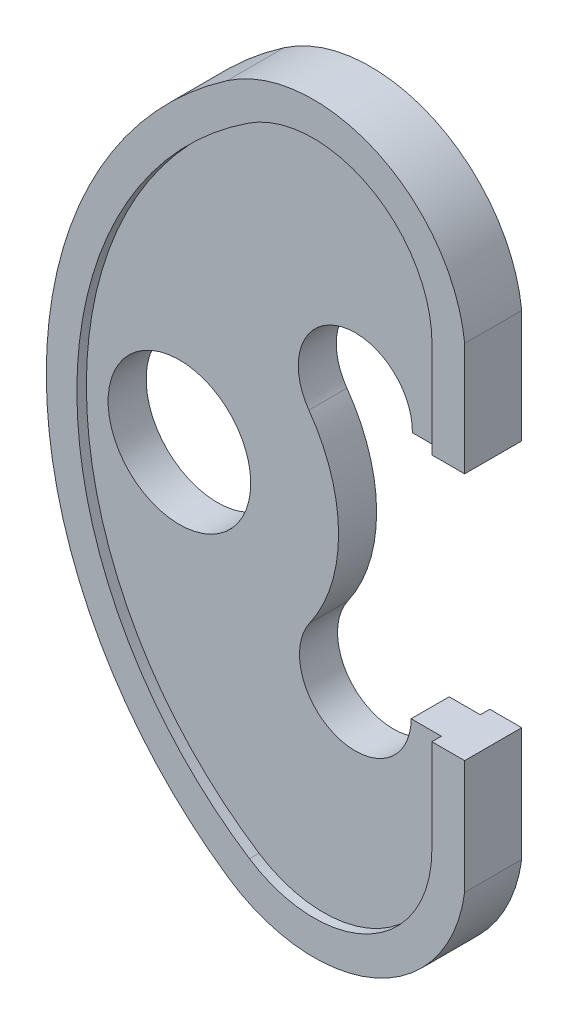
ISO-10303-21;
HEADER;
FILE_DESCRIPTION(('STEP AP214'),'2;1');
FILE_NAME('part.step','',(''),(''),'','','');
FILE_SCHEMA(('AUTOMOTIVE_DESIGN { 1 0 10303 214 1 1 1 1 }'));
ENDSEC;
DATA;
#1=APPLICATION_CONTEXT('core data for automotive mechanical design processes');
#2=APPLICATION_PROTOCOL_DEFINITION('international standard','automotive_design',2000,#1);
#3=PRODUCT_CONTEXT('',#1,'mechanical');
#4=PRODUCT('Part','Part','',(#3));
#5=PRODUCT_RELATED_PRODUCT_CATEGORY('part','',(#4));
#6=PRODUCT_DEFINITION_FORMATION('','',#4);
#7=PRODUCT_DEFINITION_CONTEXT('part definition',#1,'design');
#8=PRODUCT_DEFINITION('design','',#6,#7);
#9=PRODUCT_DEFINITION_SHAPE('','',#8);
#10=(LENGTH_UNIT() NAMED_UNIT(*) SI_UNIT(.MILLI.,.METRE.));
#11=(NAMED_UNIT(*) PLANE_ANGLE_UNIT() SI_UNIT($,.RADIAN.));
#12=(NAMED_UNIT(*) SI_UNIT($,.STERADIAN.) SOLID_ANGLE_UNIT());
#13=UNCERTAINTY_MEASURE_WITH_UNIT(LENGTH_MEASURE(1.E-05),#10,'distance_accuracy_value','');
#14=(GEOMETRIC_REPRESENTATION_CONTEXT(3) GLOBAL_UNCERTAINTY_ASSIGNED_CONTEXT((#13)) GLOBAL_UNIT_ASSIGNED_CONTEXT((#10,
#11,#12)) REPRESENTATION_CONTEXT('',''));
#15=CARTESIAN_POINT('',(0.,0.,0.));
#16=DIRECTION('',(0.,0.,1.));
#17=DIRECTION('',(1.,0.,0.));
#18=AXIS2_PLACEMENT_3D('',#15,#16,#17);
#19=CARTESIAN_POINT('',(-6.87347372301431,8.08028099134121,10.));
#20=DIRECTION('',(0.999999959439754,-0.000284816592779039,0.));
#21=DIRECTION('',(0.000284816592779039,0.999999959439754,0.));
#22=AXIS2_PLACEMENT_3D('',#19,#20,#21);
#23=PLANE('',#22);
#24=DIRECTION('',(0.000284816592779039,0.999999959439753,0.));
#25=VECTOR('',#24,1.);
#26=CARTESIAN_POINT('',(-6.87347372301431,8.08028099134121,10.));
#27=LINE('',#26,#25);
#28=CARTESIAN_POINT('',(-6.8792533227761,-12.2120744187505,10.));
#29=VERTEX_POINT('',#28);
#30=CARTESIAN_POINT('',(-6.87347372301432,8.0802809913412,10.));
#31=VERTEX_POINT('',#30);
#32=EDGE_CURVE('E361',#29,#31,#27,.T.);
#33=ORIENTED_EDGE('',*,*,#32,.F.);
#34=DIRECTION('',(0.,0.,1.));
#35=VECTOR('',#34,1.);
#36=CARTESIAN_POINT('',(-6.8792533227761,-12.2120744187505,9.99999999999997));
#37=LINE('',#36,#35);
#38=CARTESIAN_POINT('',(-6.8792533227761,-12.2120744187505,12.));
#39=VERTEX_POINT('',#38);
#40=EDGE_CURVE('E210',#29,#39,#37,.T.);
#41=ORIENTED_EDGE('',*,*,#40,.T.);
#42=DIRECTION('',(0.000284816592779039,0.999999959439753,0.));
#43=VECTOR('',#42,1.);
#44=CARTESIAN_POINT('',(-6.87347372301431,8.08028099134121,12.));
#45=LINE('',#44,#43);
#46=CARTESIAN_POINT('',(-6.87347372301432,8.0802809913412,12.));
#47=VERTEX_POINT('',#46);
#48=EDGE_CURVE('E224',#39,#47,#45,.T.);
#49=ORIENTED_EDGE('',*,*,#48,.T.);
#50=DIRECTION('',(0.,0.,1.));
#51=VECTOR('',#50,1.);
#52=CARTESIAN_POINT('',(-6.87347372301432,8.0802809913412,10.));
#53=LINE('',#52,#51);
#54=EDGE_CURVE('E234',#31,#47,#53,.T.);
#55=ORIENTED_EDGE('',*,*,#54,.F.);
#56=EDGE_LOOP('',(#33,#41,#49,#55));
#57=FACE_BOUND('',#56,.T.);
#58=ADVANCED_FACE('F50',(#57),#23,.F.);
#59=CARTESIAN_POINT('',(0.,0.,12.));
#60=DIRECTION('',(1.,0.,0.));
#61=DIRECTION('',(0.,1.,0.));
#62=AXIS2_PLACEMENT_3D('',#59,#60,#61);
#63=PLANE('',#62);
#64=DIRECTION('',(0.,-1.,0.));
#65=VECTOR('',#64,1.);
#66=CARTESIAN_POINT('',(0.,0.,12.));
#67=LINE('',#66,#65);
#68=CARTESIAN_POINT('',(0.,11.5582529857865,12.));
#69=VERTEX_POINT('',#68);
#70=CARTESIAN_POINT('',(0.,-12.2120744187505,12.));
#71=VERTEX_POINT('',#70);
#72=EDGE_CURVE('E247',#69,#71,#67,.T.);
#73=ORIENTED_EDGE('',*,*,#72,.T.);
#74=DIRECTION('',(0.,0.,1.));
#75=VECTOR('',#74,1.);
#76=CARTESIAN_POINT('',(0.,-12.2120744187505,0.));
#77=LINE('',#76,#75);
#78=CARTESIAN_POINT('',(0.,-12.2120744187505,0.));
#79=VERTEX_POINT('',#78);
#80=EDGE_CURVE('E313',#79,#71,#77,.T.);
#81=ORIENTED_EDGE('',*,*,#80,.F.);
#82=DIRECTION('',(0.,-1.,0.));
#83=VECTOR('',#82,1.);
#84=CARTESIAN_POINT('',(0.,0.,0.));
#85=LINE('',#84,#83);
#86=CARTESIAN_POINT('',(0.,11.5582529857865,0.));
#87=VERTEX_POINT('',#86);
#88=EDGE_CURVE('E262',#87,#79,#85,.T.);
#89=ORIENTED_EDGE('',*,*,#88,.F.);
#90=DIRECTION('',(0.,0.,-1.));
#91=VECTOR('',#90,1.);
#92=CARTESIAN_POINT('',(0.,11.5582529857865,12.));
#93=LINE('',#92,#91);
#94=EDGE_CURVE('E269',#69,#87,#93,.T.);
#95=ORIENTED_EDGE('',*,*,#94,.F.);
#96=EDGE_LOOP('',(#73,#81,#89,#95));
#97=FACE_BOUND('',#96,.T.);
#98=ADVANCED_FACE('F438',(#97),#63,.T.);
#99=CARTESIAN_POINT('',(-6.71169551772124,8.08738367263815,2.));
#100=DIRECTION('',(1.,0.,0.));
#101=DIRECTION('',(0.,1.,0.));
#102=AXIS2_PLACEMENT_3D('',#99,#100,#101);
#103=PLANE('',#102);
#104=DIRECTION('',(0.,-1.,0.));
#105=VECTOR('',#104,1.);
#106=CARTESIAN_POINT('',(-6.71169551772124,8.08738367263815,0.));
#107=LINE('',#106,#105);
#108=CARTESIAN_POINT('',(-6.71169551772124,8.08738367263815,0.));
#109=VERTEX_POINT('',#108);
#110=CARTESIAN_POINT('',(-6.71169551772125,-12.2120744187505,0.));
#111=VERTEX_POINT('',#110);
#112=EDGE_CURVE('E347',#109,#111,#107,.T.);
#113=ORIENTED_EDGE('',*,*,#112,.T.);
#114=DIRECTION('',(0.,0.,1.));
#115=VECTOR('',#114,1.);
#116=CARTESIAN_POINT('',(-6.71169551772125,-12.2120744187505,2.));
#117=LINE('',#116,#115);
#118=CARTESIAN_POINT('',(-6.71169551772125,-12.2120744187505,2.));
#119=VERTEX_POINT('',#118);
#120=EDGE_CURVE('E281',#111,#119,#117,.T.);
#121=ORIENTED_EDGE('',*,*,#120,.T.);
#122=DIRECTION('',(0.,-1.,0.));
#123=VECTOR('',#122,1.);
#124=CARTESIAN_POINT('',(-6.71169551772124,8.08738367263815,2.));
#125=LINE('',#124,#123);
#126=CARTESIAN_POINT('',(-6.71169551772124,8.08738367263815,2.));
#127=VERTEX_POINT('',#126);
#128=EDGE_CURVE('E333',#127,#119,#125,.T.);
#129=ORIENTED_EDGE('',*,*,#128,.F.);
#130=DIRECTION('',(0.,0.,-1.));
#131=VECTOR('',#130,1.);
#132=CARTESIAN_POINT('',(-6.71169551772124,8.08738367263815,2.));
#133=LINE('',#132,#131);
#134=EDGE_CURVE('E353',#127,#109,#133,.T.);
#135=ORIENTED_EDGE('',*,*,#134,.T.);
#136=EDGE_LOOP('',(#113,#121,#129,#135));
#137=FACE_BOUND('',#136,.T.);
#138=ADVANCED_FACE('F421',(#137),#103,.F.);
#139=CARTESIAN_POINT('',(-62.,-38.4417470142135,0.));
#140=DIRECTION('',(0.,0.,1.));
#141=DIRECTION('',(1.,0.,0.));
#142=AXIS2_PLACEMENT_3D('',#139,#140,#141);
#143=CYLINDRICAL_SURFACE('',#142,15.);
#144=CARTESIAN_POINT('',(-62.,-38.4417470142135,2.));
#145=DIRECTION('',(0.,0.,1.));
#146=DIRECTION('',(1.,0.,0.));
#147=AXIS2_PLACEMENT_3D('',#144,#145,#146);
#148=CIRCLE('',#147,15.);
#149=CARTESIAN_POINT('',(-47.,-38.4417470142135,2.));
#150=VERTEX_POINT('',#149);
#151=EDGE_CURVE('E279',#150,#150,#148,.F.);
#152=ORIENTED_EDGE('',*,*,#151,.T.);
#153=EDGE_LOOP('',(#152));
#154=FACE_BOUND('',#153,.T.);
#155=CARTESIAN_POINT('',(-62.,-38.4417470142135,10.));
#156=DIRECTION('',(0.,0.,1.));
#157=DIRECTION('',(1.,0.,0.));
#158=AXIS2_PLACEMENT_3D('',#155,#156,#157);
#159=CIRCLE('',#158,15.);
#160=CARTESIAN_POINT('',(-47.,-38.4417470142135,10.));
#161=VERTEX_POINT('',#160);
#162=EDGE_CURVE('E231',#161,#161,#159,.F.);
#163=ORIENTED_EDGE('',*,*,#162,.F.);
#164=EDGE_LOOP('',(#163));
#165=FACE_BOUND('',#164,.T.);
#166=ADVANCED_FACE('F594',(#154,#165),#143,.F.);
#167=CARTESIAN_POINT('',(0.,-38.,12.));
#168=DIRECTION('',(0.,0.,-1.));
#169=DIRECTION('',(-1.,0.,0.));
#170=AXIS2_PLACEMENT_3D('',#167,#168,#169);
#171=CYLINDRICAL_SURFACE('',#170,88.);
#172=CARTESIAN_POINT('',(0.,-38.,0.));
#173=DIRECTION('',(0.,0.,1.));
#174=DIRECTION('',(1.,0.,0.));
#175=AXIS2_PLACEMENT_3D('',#172,#173,#174);
#176=CIRCLE('',#175,88.);
#177=CARTESIAN_POINT('',(-49.9890439040348,34.4230314855742,0.));
#178=VERTEX_POINT('',#177);
#179=CARTESIAN_POINT('',(-49.8326643849906,-110.530721492985,0.));
#180=VERTEX_POINT('',#179);
#181=EDGE_CURVE('E251',#178,#180,#176,.T.);
#182=ORIENTED_EDGE('',*,*,#181,.T.);
#183=DIRECTION('',(0.,0.,-1.));
#184=VECTOR('',#183,1.);
#185=CARTESIAN_POINT('',(-49.8326643849906,-110.530721492985,12.));
#186=LINE('',#185,#184);
#187=CARTESIAN_POINT('',(-49.8326643849906,-110.530721492985,12.));
#188=VERTEX_POINT('',#187);
#189=EDGE_CURVE('E275',#188,#180,#186,.T.);
#190=ORIENTED_EDGE('',*,*,#189,.F.);
#191=CARTESIAN_POINT('',(0.,-38.,12.));
#192=DIRECTION('',(0.,0.,1.));
#193=DIRECTION('',(1.,0.,0.));
#194=AXIS2_PLACEMENT_3D('',#191,#192,#193);
#195=CIRCLE('',#194,88.);
#196=CARTESIAN_POINT('',(-49.9890439040348,34.4230314855742,12.));
#197=VERTEX_POINT('',#196);
#198=EDGE_CURVE('E245',#197,#188,#195,.T.);
#199=ORIENTED_EDGE('',*,*,#198,.F.);
#200=DIRECTION('',(0.,0.,-1.));
#201=VECTOR('',#200,1.);
#202=CARTESIAN_POINT('',(-49.9890439040348,34.4230314855742,12.));
#203=LINE('',#202,#201);
#204=EDGE_CURVE('E254',#197,#178,#203,.T.);
#205=ORIENTED_EDGE('',*,*,#204,.T.);
#206=EDGE_LOOP('',(#182,#190,#199,#205));
#207=FACE_BOUND('',#206,.T.);
#208=ADVANCED_FACE('F47',(#207),#171,.T.);
#209=CARTESIAN_POINT('',(-31.7116955177213,-84.1559136773538,12.));
#210=DIRECTION('',(0.,0.,-1.));
#211=DIRECTION('',(-1.,0.,0.));
#212=AXIS2_PLACEMENT_3D('',#209,#210,#211);
#213=CYLINDRICAL_SURFACE('',#212,32.);
#214=CARTESIAN_POINT('',(-31.7116955177213,-84.1559136773538,0.));
#215=DIRECTION('',(0.,0.,1.));
#216=DIRECTION('',(1.,0.,0.));
#217=AXIS2_PLACEMENT_3D('',#214,#215,#216);
#218=CIRCLE('',#217,32.);
#219=CARTESIAN_POINT('',(0.,-88.4417470142135,0.));
#220=VERTEX_POINT('',#219);
#221=EDGE_CURVE('E260',#180,#220,#218,.T.);
#222=ORIENTED_EDGE('',*,*,#221,.T.);
#223=DIRECTION('',(0.,0.,-1.));
#224=VECTOR('',#223,1.);
#225=CARTESIAN_POINT('',(0.,-88.4417470142135,12.));
#226=LINE('',#225,#224);
#227=CARTESIAN_POINT('',(0.,-88.4417470142135,12.));
#228=VERTEX_POINT('',#227);
#229=EDGE_CURVE('E266',#228,#220,#226,.T.);
#230=ORIENTED_EDGE('',*,*,#229,.F.);
#231=CARTESIAN_POINT('',(-31.7116955177213,-84.1559136773538,12.));
#232=DIRECTION('',(0.,0.,1.));
#233=DIRECTION('',(1.,0.,0.));
#234=AXIS2_PLACEMENT_3D('',#231,#232,#233);
#235=CIRCLE('',#234,32.);
#236=EDGE_CURVE('E244',#188,#228,#235,.T.);
#237=ORIENTED_EDGE('',*,*,#236,.F.);
#238=ORIENTED_EDGE('',*,*,#189,.T.);
#239=EDGE_LOOP('',(#222,#230,#237,#238));
#240=FACE_BOUND('',#239,.T.);
#241=ADVANCED_FACE('F534',(#240),#213,.T.);
#242=DIRECTION('',(0.,0.,1.));
#243=VECTOR('',#242,1.);
#244=CARTESIAN_POINT('',(0.,-64.4417470142135,0.));
#245=LINE('',#244,#243);
#246=CARTESIAN_POINT('',(0.,-64.4417470142135,0.));
#247=VERTEX_POINT('',#246);
#248=CARTESIAN_POINT('',(0.,-64.4417470142135,12.));
#249=VERTEX_POINT('',#248);
#250=EDGE_CURVE('E316',#247,#249,#245,.T.);
#251=ORIENTED_EDGE('',*,*,#250,.T.);
#252=EDGE_CURVE('E203',#249,#228,#67,.T.);
#253=ORIENTED_EDGE('',*,*,#252,.T.);
#254=ORIENTED_EDGE('',*,*,#229,.T.);
#255=EDGE_CURVE('E258',#247,#220,#85,.T.);
#256=ORIENTED_EDGE('',*,*,#255,.F.);
#257=EDGE_LOOP('',(#251,#253,#254,#256));
#258=FACE_BOUND('',#257,.T.);
#259=ADVANCED_FACE('F447',(#258),#63,.T.);
#260=CARTESIAN_POINT('',(-31.8112097571131,8.08738367263816,12.));
#261=DIRECTION('',(0.,0.,-1.));
#262=DIRECTION('',(-1.,0.,0.));
#263=AXIS2_PLACEMENT_3D('',#260,#261,#262);
#264=CYLINDRICAL_SURFACE('',#263,32.);
#265=CARTESIAN_POINT('',(-31.8112097571131,8.08738367263816,0.));
#266=DIRECTION('',(0.,0.,1.));
#267=DIRECTION('',(1.,0.,0.));
#268=AXIS2_PLACEMENT_3D('',#265,#266,#267);
#269=CIRCLE('',#268,32.);
#270=EDGE_CURVE('E246',#87,#178,#269,.T.);
#271=ORIENTED_EDGE('',*,*,#270,.T.);
#272=ORIENTED_EDGE('',*,*,#204,.F.);
#273=CARTESIAN_POINT('',(-31.8112097571131,8.08738367263816,12.));
#274=DIRECTION('',(0.,0.,1.));
#275=DIRECTION('',(1.,0.,0.));
#276=AXIS2_PLACEMENT_3D('',#273,#274,#275);
#277=CIRCLE('',#276,32.);
#278=EDGE_CURVE('E252',#69,#197,#277,.T.);
#279=ORIENTED_EDGE('',*,*,#278,.F.);
#280=ORIENTED_EDGE('',*,*,#94,.T.);
#281=EDGE_LOOP('',(#271,#272,#279,#280));
#282=FACE_BOUND('',#281,.T.);
#283=ADVANCED_FACE('F519',(#282),#264,.T.);
#284=CARTESIAN_POINT('',(0.,0.,12.));
#285=DIRECTION('',(0.,0.,1.));
#286=DIRECTION('',(1.,0.,0.));
#287=AXIS2_PLACEMENT_3D('',#284,#285,#286);
#288=PLANE('',#287);
#289=ORIENTED_EDGE('',*,*,#48,.F.);
#290=DIRECTION('',(-1.,0.,0.));
#291=VECTOR('',#290,1.);
#292=CARTESIAN_POINT('',(0.,-12.2120744187505,12.));
#293=LINE('',#292,#291);
#294=EDGE_CURVE('E207',#71,#39,#293,.T.);
#295=ORIENTED_EDGE('',*,*,#294,.F.);
#296=ORIENTED_EDGE('',*,*,#72,.F.);
#297=ORIENTED_EDGE('',*,*,#278,.T.);
#298=ORIENTED_EDGE('',*,*,#198,.T.);
#299=ORIENTED_EDGE('',*,*,#236,.T.);
#300=ORIENTED_EDGE('',*,*,#252,.F.);
#301=DIRECTION('',(1.,0.,0.));
#302=VECTOR('',#301,1.);
#303=CARTESIAN_POINT('',(0.,-64.4417470142135,12.));
#304=LINE('',#303,#302);
#305=CARTESIAN_POINT('',(-6.89412920077007,-64.4417470142135,12.));
#306=VERTEX_POINT('',#305);
#307=EDGE_CURVE('E200',#306,#249,#304,.T.);
#308=ORIENTED_EDGE('',*,*,#307,.F.);
#309=CARTESIAN_POINT('',(-6.89974613553398,-84.1629805325237,12.));
#310=VERTEX_POINT('',#309);
#311=EDGE_CURVE('E205',#310,#306,#45,.T.);
#312=ORIENTED_EDGE('',*,*,#311,.F.);
#313=CARTESIAN_POINT('',(-31.7116955177213,-84.1559136773538,12.));
#314=DIRECTION('',(0.,0.,1.));
#315=DIRECTION('',(1.,0.,0.));
#316=AXIS2_PLACEMENT_3D('',#313,#314,#315);
#317=CIRCLE('',#316,24.8119503885661);
#318=CARTESIAN_POINT('',(-45.2633918891372,-104.940148268544,12.));
#319=VERTEX_POINT('',#318);
#320=EDGE_CURVE('E227',#319,#310,#317,.T.);
#321=ORIENTED_EDGE('',*,*,#320,.F.);
#322=CARTESIAN_POINT('',(-1.56929719947238,-37.9265221224338,12.));
#323=DIRECTION('',(0.,0.,1.));
#324=DIRECTION('',(1.,0.,0.));
#325=AXIS2_PLACEMENT_3D('',#322,#323,#324);
#326=CIRCLE('',#325,79.9999999999999);
#327=CARTESIAN_POINT('',(-45.5077929095733,28.9271134909974,12.));
#328=VERTEX_POINT('',#327);
#329=EDGE_CURVE('E282',#328,#319,#326,.T.);
#330=ORIENTED_EDGE('',*,*,#329,.F.);
#331=CARTESIAN_POINT('',(-31.8112097571131,8.08738367263816,12.));
#332=DIRECTION('',(0.,0.,1.));
#333=DIRECTION('',(1.,0.,0.));
#334=AXIS2_PLACEMENT_3D('',#331,#332,#333);
#335=CIRCLE('',#334,24.9377370455795);
#336=EDGE_CURVE('E222',#47,#328,#335,.T.);
#337=ORIENTED_EDGE('',*,*,#336,.F.);
#338=EDGE_LOOP('',(#289,#295,#296,#297,#298,#299,#300,#308,#312,#321,#330,#337));
#339=FACE_BOUND('',#338,.T.);
#340=ADVANCED_FACE('F198',(#339),#288,.T.);
#341=CARTESIAN_POINT('',(0.,0.,0.));
#342=DIRECTION('',(0.,0.,1.));
#343=DIRECTION('',(1.,0.,0.));
#344=AXIS2_PLACEMENT_3D('',#341,#342,#343);
#345=PLANE('',#344);
#346=ORIENTED_EDGE('',*,*,#88,.T.);
#347=DIRECTION('',(-1.,0.,0.));
#348=VECTOR('',#347,1.);
#349=CARTESIAN_POINT('',(0.,-12.2120744187505,0.));
#350=LINE('',#349,#348);
#351=EDGE_CURVE('E324',#79,#111,#350,.T.);
#352=ORIENTED_EDGE('',*,*,#351,.T.);
#353=ORIENTED_EDGE('',*,*,#112,.F.);
#354=CARTESIAN_POINT('',(-31.8112097571131,8.08738367263816,0.));
#355=DIRECTION('',(0.,0.,-1.));
#356=DIRECTION('',(-1.,0.,0.));
#357=AXIS2_PLACEMENT_3D('',#354,#355,#356);
#358=CIRCLE('',#357,25.0995142393918);
#359=CARTESIAN_POINT('',(-45.4907300450156,29.1315358234447,0.));
#360=VERTEX_POINT('',#359);
#361=EDGE_CURVE('E345',#360,#109,#358,.T.);
#362=ORIENTED_EDGE('',*,*,#361,.F.);
#363=CARTESIAN_POINT('',(-1.88982157346105,-37.9427571691402,0.));
#364=DIRECTION('',(0.,0.,-1.));
#365=DIRECTION('',(1.,0.,0.));
#366=AXIS2_PLACEMENT_3D('',#363,#364,#365);
#367=CIRCLE('',#366,80.);
#368=CARTESIAN_POINT('',(-45.2670927651123,-105.16189390836,0.));
#369=VERTEX_POINT('',#368);
#370=EDGE_CURVE('E68',#369,#360,#367,.T.);
#371=ORIENTED_EDGE('',*,*,#370,.F.);
#372=CARTESIAN_POINT('',(-31.7116955177213,-84.1559136773538,0.));
#373=DIRECTION('',(0.,0.,-1.));
#374=DIRECTION('',(-1.,0.,0.));
#375=AXIS2_PLACEMENT_3D('',#372,#373,#374);
#376=CIRCLE('',#375,25.);
#377=CARTESIAN_POINT('',(-6.71169551772124,-84.1559136773538,0.));
#378=VERTEX_POINT('',#377);
#379=EDGE_CURVE('E332',#378,#369,#376,.T.);
#380=ORIENTED_EDGE('',*,*,#379,.F.);
#381=CARTESIAN_POINT('',(-6.71169551772125,-64.4417470142135,0.));
#382=VERTEX_POINT('',#381);
#383=EDGE_CURVE('E343',#382,#378,#107,.T.);
#384=ORIENTED_EDGE('',*,*,#383,.F.);
#385=DIRECTION('',(1.,0.,0.));
#386=VECTOR('',#385,1.);
#387=CARTESIAN_POINT('',(-13.25855129318,-64.4417470142135,0.));
#388=LINE('',#387,#386);
#389=EDGE_CURVE('E65',#382,#247,#388,.T.);
#390=ORIENTED_EDGE('',*,*,#389,.T.);
#391=ORIENTED_EDGE('',*,*,#255,.T.);
#392=ORIENTED_EDGE('',*,*,#221,.F.);
#393=ORIENTED_EDGE('',*,*,#181,.F.);
#394=ORIENTED_EDGE('',*,*,#270,.F.);
#395=EDGE_LOOP('',(#346,#352,#353,#362,#371,#380,#384,#390,#391,#392,#393,#394));
#396=FACE_BOUND('',#395,.T.);
#397=ADVANCED_FACE('F433',(#396),#345,.F.);
#398=CARTESIAN_POINT('',(-1.56929719947238,-37.9265221224338,10.));
#399=DIRECTION('',(0.,0.,1.));
#400=DIRECTION('',(1.,0.,0.));
#401=AXIS2_PLACEMENT_3D('',#398,#399,#400);
#402=PLANE('',#401);
#403=DIRECTION('',(-1.,0.,0.));
#404=VECTOR('',#403,1.);
#405=CARTESIAN_POINT('',(-12.9979710146966,-12.2120744187505,10.));
#406=LINE('',#405,#404);
#407=CARTESIAN_POINT('',(-12.9979710146966,-12.2120744187505,10.));
#408=VERTEX_POINT('',#407);
#409=EDGE_CURVE('E397',#29,#408,#406,.T.);
#410=ORIENTED_EDGE('',*,*,#409,.F.);
#411=ORIENTED_EDGE('',*,*,#32,.T.);
#412=CARTESIAN_POINT('',(-31.8112097571131,8.08738367263816,10.));
#413=DIRECTION('',(0.,0.,1.));
#414=DIRECTION('',(1.,0.,0.));
#415=AXIS2_PLACEMENT_3D('',#412,#413,#414);
#416=CIRCLE('',#415,24.9377370455795);
#417=CARTESIAN_POINT('',(-45.5077929095733,28.9271134909974,10.));
#418=VERTEX_POINT('',#417);
#419=EDGE_CURVE('E241',#31,#418,#416,.T.);
#420=ORIENTED_EDGE('',*,*,#419,.T.);
#421=CARTESIAN_POINT('',(-1.56929719947238,-37.9265221224338,10.));
#422=DIRECTION('',(0.,0.,1.));
#423=DIRECTION('',(1.,0.,0.));
#424=AXIS2_PLACEMENT_3D('',#421,#422,#423);
#425=CIRCLE('',#424,79.9999999999999);
#426=CARTESIAN_POINT('',(-45.2633918891372,-104.940148268544,10.));
#427=VERTEX_POINT('',#426);
#428=EDGE_CURVE('E223',#418,#427,#425,.T.);
#429=ORIENTED_EDGE('',*,*,#428,.T.);
#430=CARTESIAN_POINT('',(-31.7116955177213,-84.1559136773538,10.));
#431=DIRECTION('',(0.,0.,1.));
#432=DIRECTION('',(1.,0.,0.));
#433=AXIS2_PLACEMENT_3D('',#430,#431,#432);
#434=CIRCLE('',#433,24.8119503885661);
#435=CARTESIAN_POINT('',(-6.89974613553398,-84.1629805325237,10.));
#436=VERTEX_POINT('',#435);
#437=EDGE_CURVE('E359',#427,#436,#434,.T.);
#438=ORIENTED_EDGE('',*,*,#437,.T.);
#439=CARTESIAN_POINT('',(-6.89412920077007,-64.4417470142135,10.));
#440=VERTEX_POINT('',#439);
#441=EDGE_CURVE('E364',#436,#440,#27,.T.);
#442=ORIENTED_EDGE('',*,*,#441,.T.);
#443=DIRECTION('',(1.,0.,0.));
#444=VECTOR('',#443,1.);
#445=CARTESIAN_POINT('',(-6.89412920077007,-64.4417470142135,10.));
#446=LINE('',#445,#444);
#447=CARTESIAN_POINT('',(-13.25855129318,-64.4417470142135,10.));
#448=VERTEX_POINT('',#447);
#449=EDGE_CURVE('E214',#448,#440,#446,.T.);
#450=ORIENTED_EDGE('',*,*,#449,.F.);
#451=CARTESIAN_POINT('',(-25.,-64.4417470142135,10.));
#452=DIRECTION('',(0.,0.,1.));
#453=DIRECTION('',(1.,0.,0.));
#454=AXIS2_PLACEMENT_3D('',#451,#452,#453);
#455=CIRCLE('',#454,11.74144870682);
#456=CARTESIAN_POINT('',(-34.6067558410355,-57.6910537205129,10.));
#457=VERTEX_POINT('',#456);
#458=EDGE_CURVE('E389',#457,#448,#455,.T.);
#459=ORIENTED_EDGE('',*,*,#458,.F.);
#460=CARTESIAN_POINT('',(-62.,-38.4417470142135,10.));
#461=DIRECTION('',(0.,0.,-1.));
#462=DIRECTION('',(1.,0.,0.));
#463=AXIS2_PLACEMENT_3D('',#460,#461,#462);
#464=CIRCLE('',#463,33.4802275115601);
#465=CARTESIAN_POINT('',(-34.7596117688961,-18.9767301058068,10.));
#466=VERTEX_POINT('',#465);
#467=EDGE_CURVE('E388',#466,#457,#464,.T.);
#468=ORIENTED_EDGE('',*,*,#467,.F.);
#469=CARTESIAN_POINT('',(-24.9960981051858,-12.0000689460154,10.));
#470=DIRECTION('',(0.,0.,1.));
#471=DIRECTION('',(1.,0.,0.));
#472=AXIS2_PLACEMENT_3D('',#469,#470,#471);
#473=CIRCLE('',#472,12.);
#474=EDGE_CURVE('E308',#408,#466,#473,.T.);
#475=ORIENTED_EDGE('',*,*,#474,.F.);
#476=EDGE_LOOP('',(#410,#411,#420,#429,#438,#442,#450,#459,#468,#475));
#477=FACE_BOUND('',#476,.T.);
#478=ORIENTED_EDGE('',*,*,#162,.T.);
#479=EDGE_LOOP('',(#478));
#480=FACE_BOUND('',#479,.T.);
#481=ADVANCED_FACE('F398',(#477,#480),#402,.T.);
#482=CARTESIAN_POINT('',(-1.56929719947238,-37.9265221224338,10.));
#483=DIRECTION('',(0.,0.,1.));
#484=DIRECTION('',(1.,0.,0.));
#485=AXIS2_PLACEMENT_3D('',#482,#483,#484);
#486=CYLINDRICAL_SURFACE('',#485,79.9999999999999);
#487=ORIENTED_EDGE('',*,*,#329,.T.);
#488=DIRECTION('',(0.,0.,1.));
#489=VECTOR('',#488,1.);
#490=CARTESIAN_POINT('',(-45.2633918891372,-104.940148268544,10.));
#491=LINE('',#490,#489);
#492=EDGE_CURVE('E238',#427,#319,#491,.T.);
#493=ORIENTED_EDGE('',*,*,#492,.F.);
#494=ORIENTED_EDGE('',*,*,#428,.F.);
#495=DIRECTION('',(0.,0.,1.));
#496=VECTOR('',#495,1.);
#497=CARTESIAN_POINT('',(-45.5077929095733,28.9271134909974,10.));
#498=LINE('',#497,#496);
#499=EDGE_CURVE('E233',#418,#328,#498,.T.);
#500=ORIENTED_EDGE('',*,*,#499,.T.);
#501=EDGE_LOOP('',(#487,#493,#494,#500));
#502=FACE_BOUND('',#501,.T.);
#503=ADVANCED_FACE('F424',(#502),#486,.F.);
#504=CARTESIAN_POINT('',(-31.8112097571131,8.08738367263816,10.));
#505=DIRECTION('',(0.,0.,1.));
#506=DIRECTION('',(1.,0.,0.));
#507=AXIS2_PLACEMENT_3D('',#504,#505,#506);
#508=CYLINDRICAL_SURFACE('',#507,24.9377370455795);
#509=ORIENTED_EDGE('',*,*,#336,.T.);
#510=ORIENTED_EDGE('',*,*,#499,.F.);
#511=ORIENTED_EDGE('',*,*,#419,.F.);
#512=ORIENTED_EDGE('',*,*,#54,.T.);
#513=EDGE_LOOP('',(#509,#510,#511,#512));
#514=FACE_BOUND('',#513,.T.);
#515=ADVANCED_FACE('F374',(#514),#508,.F.);
#516=ORIENTED_EDGE('',*,*,#311,.T.);
#517=DIRECTION('',(0.,0.,-1.));
#518=VECTOR('',#517,1.);
#519=CARTESIAN_POINT('',(-6.89412920077007,-64.4417470142135,10.));
#520=LINE('',#519,#518);
#521=EDGE_CURVE('E208',#306,#440,#520,.T.);
#522=ORIENTED_EDGE('',*,*,#521,.T.);
#523=ORIENTED_EDGE('',*,*,#441,.F.);
#524=DIRECTION('',(0.,0.,1.));
#525=VECTOR('',#524,1.);
#526=CARTESIAN_POINT('',(-6.89974613553398,-84.1629805325237,10.));
#527=LINE('',#526,#525);
#528=EDGE_CURVE('E216',#436,#310,#527,.T.);
#529=ORIENTED_EDGE('',*,*,#528,.T.);
#530=EDGE_LOOP('',(#516,#522,#523,#529));
#531=FACE_BOUND('',#530,.T.);
#532=ADVANCED_FACE('F219',(#531),#23,.F.);
#533=CARTESIAN_POINT('',(-31.7116955177213,-84.1559136773538,10.));
#534=DIRECTION('',(0.,0.,1.));
#535=DIRECTION('',(1.,0.,0.));
#536=AXIS2_PLACEMENT_3D('',#533,#534,#535);
#537=CYLINDRICAL_SURFACE('',#536,24.8119503885661);
#538=ORIENTED_EDGE('',*,*,#320,.T.);
#539=ORIENTED_EDGE('',*,*,#528,.F.);
#540=ORIENTED_EDGE('',*,*,#437,.F.);
#541=ORIENTED_EDGE('',*,*,#492,.T.);
#542=EDGE_LOOP('',(#538,#539,#540,#541));
#543=FACE_BOUND('',#542,.T.);
#544=ADVANCED_FACE('F369',(#543),#537,.F.);
#545=CARTESIAN_POINT('',(-1.88982157346105,-37.9427571691402,2.));
#546=DIRECTION('',(0.,0.,1.));
#547=DIRECTION('',(1.,0.,0.));
#548=AXIS2_PLACEMENT_3D('',#545,#546,#547);
#549=PLANE('',#548);
#550=ORIENTED_EDGE('',*,*,#128,.T.);
#551=DIRECTION('',(-1.,0.,0.));
#552=VECTOR('',#551,1.);
#553=CARTESIAN_POINT('',(-1.88982157346103,-12.2120744187505,2.));
#554=LINE('',#553,#552);
#555=CARTESIAN_POINT('',(-12.9979710146966,-12.2120744187505,2.));
#556=VERTEX_POINT('',#555);
#557=EDGE_CURVE('E323',#119,#556,#554,.T.);
#558=ORIENTED_EDGE('',*,*,#557,.T.);
#559=CARTESIAN_POINT('',(-24.9960981051858,-12.0000689460154,2.));
#560=DIRECTION('',(0.,0.,1.));
#561=DIRECTION('',(1.,0.,0.));
#562=AXIS2_PLACEMENT_3D('',#559,#560,#561);
#563=CIRCLE('',#562,12.);
#564=CARTESIAN_POINT('',(-34.7596117688961,-18.9767301058068,2.));
#565=VERTEX_POINT('',#564);
#566=EDGE_CURVE('E11',#556,#565,#563,.T.);
#567=ORIENTED_EDGE('',*,*,#566,.T.);
#568=CARTESIAN_POINT('',(-62.,-38.4417470142135,2.));
#569=DIRECTION('',(0.,0.,1.));
#570=DIRECTION('',(1.,0.,0.));
#571=AXIS2_PLACEMENT_3D('',#568,#569,#570);
#572=CIRCLE('',#571,33.4802275115601);
#573=CARTESIAN_POINT('',(-34.6067558410355,-57.6910537205129,2.));
#574=VERTEX_POINT('',#573);
#575=EDGE_CURVE('E54',#565,#574,#572,.F.);
#576=ORIENTED_EDGE('',*,*,#575,.T.);
#577=CARTESIAN_POINT('',(-25.,-64.4417470142135,2.));
#578=DIRECTION('',(0.,0.,1.));
#579=DIRECTION('',(1.,0.,0.));
#580=AXIS2_PLACEMENT_3D('',#577,#578,#579);
#581=CIRCLE('',#580,11.74144870682);
#582=CARTESIAN_POINT('',(-13.25855129318,-64.4417470142135,2.));
#583=VERTEX_POINT('',#582);
#584=EDGE_CURVE('E289',#574,#583,#581,.T.);
#585=ORIENTED_EDGE('',*,*,#584,.T.);
#586=DIRECTION('',(1.,0.,0.));
#587=VECTOR('',#586,1.);
#588=CARTESIAN_POINT('',(-1.88982157346105,-64.4417470142135,2.));
#589=LINE('',#588,#587);
#590=CARTESIAN_POINT('',(-6.71169551772125,-64.4417470142135,2.));
#591=VERTEX_POINT('',#590);
#592=EDGE_CURVE('E315',#583,#591,#589,.T.);
#593=ORIENTED_EDGE('',*,*,#592,.T.);
#594=CARTESIAN_POINT('',(-6.71169551772124,-84.1559136773538,2.));
#595=VERTEX_POINT('',#594);
#596=EDGE_CURVE('E331',#591,#595,#125,.T.);
#597=ORIENTED_EDGE('',*,*,#596,.T.);
#598=CARTESIAN_POINT('',(-31.7116955177213,-84.1559136773538,2.));
#599=DIRECTION('',(0.,0.,-1.));
#600=DIRECTION('',(-1.,0.,0.));
#601=AXIS2_PLACEMENT_3D('',#598,#599,#600);
#602=CIRCLE('',#601,25.);
#603=CARTESIAN_POINT('',(-45.2670927651123,-105.16189390836,2.));
#604=VERTEX_POINT('',#603);
#605=EDGE_CURVE('E340',#595,#604,#602,.T.);
#606=ORIENTED_EDGE('',*,*,#605,.T.);
#607=CARTESIAN_POINT('',(-1.88982157346105,-37.9427571691402,2.));
#608=DIRECTION('',(0.,0.,-1.));
#609=DIRECTION('',(1.,0.,0.));
#610=AXIS2_PLACEMENT_3D('',#607,#608,#609);
#611=CIRCLE('',#610,80.);
#612=CARTESIAN_POINT('',(-45.4907300450156,29.1315358234447,2.));
#613=VERTEX_POINT('',#612);
#614=EDGE_CURVE('E330',#604,#613,#611,.T.);
#615=ORIENTED_EDGE('',*,*,#614,.T.);
#616=CARTESIAN_POINT('',(-31.8112097571131,8.08738367263816,2.));
#617=DIRECTION('',(0.,0.,-1.));
#618=DIRECTION('',(-1.,0.,0.));
#619=AXIS2_PLACEMENT_3D('',#616,#617,#618);
#620=CIRCLE('',#619,25.0995142393918);
#621=EDGE_CURVE('E328',#613,#127,#620,.T.);
#622=ORIENTED_EDGE('',*,*,#621,.T.);
#623=EDGE_LOOP('',(#550,#558,#567,#576,#585,#593,#597,#606,#615,#622));
#624=FACE_BOUND('',#623,.T.);
#625=ORIENTED_EDGE('',*,*,#151,.F.);
#626=EDGE_LOOP('',(#625));
#627=FACE_BOUND('',#626,.T.);
#628=ADVANCED_FACE('F292',(#624,#627),#549,.F.);
#629=CARTESIAN_POINT('',(-1.88982157346105,-37.9427571691402,2.));
#630=DIRECTION('',(0.,0.,-1.));
#631=DIRECTION('',(-1.,0.,0.));
#632=AXIS2_PLACEMENT_3D('',#629,#630,#631);
#633=CYLINDRICAL_SURFACE('',#632,80.);
#634=ORIENTED_EDGE('',*,*,#370,.T.);
#635=DIRECTION('',(0.,0.,-1.));
#636=VECTOR('',#635,1.);
#637=CARTESIAN_POINT('',(-45.4907300450156,29.1315358234447,2.));
#638=LINE('',#637,#636);
#639=EDGE_CURVE('E338',#613,#360,#638,.T.);
#640=ORIENTED_EDGE('',*,*,#639,.F.);
#641=ORIENTED_EDGE('',*,*,#614,.F.);
#642=DIRECTION('',(0.,0.,-1.));
#643=VECTOR('',#642,1.);
#644=CARTESIAN_POINT('',(-45.2670927651123,-105.16189390836,2.));
#645=LINE('',#644,#643);
#646=EDGE_CURVE('E285',#604,#369,#645,.T.);
#647=ORIENTED_EDGE('',*,*,#646,.T.);
#648=EDGE_LOOP('',(#634,#640,#641,#647));
#649=FACE_BOUND('',#648,.T.);
#650=ADVANCED_FACE('F417',(#649),#633,.F.);
#651=CARTESIAN_POINT('',(-31.7116955177213,-84.1559136773538,2.));
#652=DIRECTION('',(0.,0.,-1.));
#653=DIRECTION('',(-1.,0.,0.));
#654=AXIS2_PLACEMENT_3D('',#651,#652,#653);
#655=CYLINDRICAL_SURFACE('',#654,25.);
#656=ORIENTED_EDGE('',*,*,#379,.T.);
#657=ORIENTED_EDGE('',*,*,#646,.F.);
#658=ORIENTED_EDGE('',*,*,#605,.F.);
#659=DIRECTION('',(0.,0.,-1.));
#660=VECTOR('',#659,1.);
#661=CARTESIAN_POINT('',(-6.71169551772124,-84.1559136773538,2.));
#662=LINE('',#661,#660);
#663=EDGE_CURVE('E354',#595,#378,#662,.T.);
#664=ORIENTED_EDGE('',*,*,#663,.T.);
#665=EDGE_LOOP('',(#656,#657,#658,#664));
#666=FACE_BOUND('',#665,.T.);
#667=ADVANCED_FACE('F414',(#666),#655,.F.);
#668=ORIENTED_EDGE('',*,*,#596,.F.);
#669=DIRECTION('',(0.,0.,-1.));
#670=VECTOR('',#669,1.);
#671=CARTESIAN_POINT('',(-6.71169551772125,-64.4417470142135,2.));
#672=LINE('',#671,#670);
#673=EDGE_CURVE('E273',#591,#382,#672,.T.);
#674=ORIENTED_EDGE('',*,*,#673,.T.);
#675=ORIENTED_EDGE('',*,*,#383,.T.);
#676=ORIENTED_EDGE('',*,*,#663,.F.);
#677=EDGE_LOOP('',(#668,#674,#675,#676));
#678=FACE_BOUND('',#677,.T.);
#679=ADVANCED_FACE('F409',(#678),#103,.F.);
#680=CARTESIAN_POINT('',(-31.8112097571131,8.08738367263816,2.));
#681=DIRECTION('',(0.,0.,-1.));
#682=DIRECTION('',(-1.,0.,0.));
#683=AXIS2_PLACEMENT_3D('',#680,#681,#682);
#684=CYLINDRICAL_SURFACE('',#683,25.0995142393918);
#685=ORIENTED_EDGE('',*,*,#361,.T.);
#686=ORIENTED_EDGE('',*,*,#134,.F.);
#687=ORIENTED_EDGE('',*,*,#621,.F.);
#688=ORIENTED_EDGE('',*,*,#639,.T.);
#689=EDGE_LOOP('',(#685,#686,#687,#688));
#690=FACE_BOUND('',#689,.T.);
#691=ADVANCED_FACE('F416',(#690),#684,.F.);
#692=CARTESIAN_POINT('',(-25.,-64.4417470142135,0.));
#693=DIRECTION('',(0.,0.,1.));
#694=DIRECTION('',(1.,0.,0.));
#695=AXIS2_PLACEMENT_3D('',#692,#693,#694);
#696=CYLINDRICAL_SURFACE('',#695,11.74144870682);
#697=DIRECTION('',(0.,0.,1.));
#698=VECTOR('',#697,1.);
#699=CARTESIAN_POINT('',(-34.6067558410355,-57.6910537205129,0.));
#700=LINE('',#699,#698);
#701=EDGE_CURVE('E303',#574,#457,#700,.T.);
#702=ORIENTED_EDGE('',*,*,#701,.T.);
#703=ORIENTED_EDGE('',*,*,#458,.T.);
#704=DIRECTION('',(0.,0.,1.));
#705=VECTOR('',#704,1.);
#706=CARTESIAN_POINT('',(-13.25855129318,-64.4417470142135,0.));
#707=LINE('',#706,#705);
#708=EDGE_CURVE('E322',#583,#448,#707,.T.);
#709=ORIENTED_EDGE('',*,*,#708,.F.);
#710=ORIENTED_EDGE('',*,*,#584,.F.);
#711=EDGE_LOOP('',(#702,#703,#709,#710));
#712=FACE_BOUND('',#711,.T.);
#713=ADVANCED_FACE('F404',(#712),#696,.F.);
#714=CARTESIAN_POINT('',(-62.,-38.4417470142135,0.));
#715=DIRECTION('',(0.,0.,1.));
#716=DIRECTION('',(1.,0.,0.));
#717=AXIS2_PLACEMENT_3D('',#714,#715,#716);
#718=CYLINDRICAL_SURFACE('',#717,33.4802275115601);
#719=DIRECTION('',(0.,0.,1.));
#720=VECTOR('',#719,1.);
#721=CARTESIAN_POINT('',(-34.7596117688961,-18.9767301058068,0.));
#722=LINE('',#721,#720);
#723=EDGE_CURVE('E301',#565,#466,#722,.T.);
#724=ORIENTED_EDGE('',*,*,#723,.T.);
#725=ORIENTED_EDGE('',*,*,#467,.T.);
#726=ORIENTED_EDGE('',*,*,#701,.F.);
#727=ORIENTED_EDGE('',*,*,#575,.F.);
#728=EDGE_LOOP('',(#724,#725,#726,#727));
#729=FACE_BOUND('',#728,.T.);
#730=ADVANCED_FACE('F299',(#729),#718,.T.);
#731=CARTESIAN_POINT('',(-24.9960981051858,-12.0000689460154,0.));
#732=DIRECTION('',(0.,0.,1.));
#733=DIRECTION('',(1.,0.,0.));
#734=AXIS2_PLACEMENT_3D('',#731,#732,#733);
#735=CYLINDRICAL_SURFACE('',#734,12.);
#736=DIRECTION('',(0.,0.,1.));
#737=VECTOR('',#736,1.);
#738=CARTESIAN_POINT('',(-12.9979710146966,-12.2120744187505,0.));
#739=LINE('',#738,#737);
#740=EDGE_CURVE('E309',#556,#408,#739,.T.);
#741=ORIENTED_EDGE('',*,*,#740,.T.);
#742=ORIENTED_EDGE('',*,*,#474,.T.);
#743=ORIENTED_EDGE('',*,*,#723,.F.);
#744=ORIENTED_EDGE('',*,*,#566,.F.);
#745=EDGE_LOOP('',(#741,#742,#743,#744));
#746=FACE_BOUND('',#745,.T.);
#747=ADVANCED_FACE('F304',(#746),#735,.F.);
#748=CARTESIAN_POINT('',(-12.9979710146966,-12.2120744187505,0.));
#749=DIRECTION('',(0.,1.,0.));
#750=DIRECTION('',(-1.,0.,0.));
#751=AXIS2_PLACEMENT_3D('',#748,#749,#750);
#752=PLANE('',#751);
#753=ORIENTED_EDGE('',*,*,#40,.F.);
#754=ORIENTED_EDGE('',*,*,#409,.T.);
#755=ORIENTED_EDGE('',*,*,#740,.F.);
#756=ORIENTED_EDGE('',*,*,#557,.F.);
#757=ORIENTED_EDGE('',*,*,#120,.F.);
#758=ORIENTED_EDGE('',*,*,#351,.F.);
#759=ORIENTED_EDGE('',*,*,#80,.T.);
#760=ORIENTED_EDGE('',*,*,#294,.T.);
#761=EDGE_LOOP('',(#753,#754,#755,#756,#757,#758,#759,#760));
#762=FACE_BOUND('',#761,.T.);
#763=ADVANCED_FACE('F425',(#762),#752,.F.);
#764=CARTESIAN_POINT('',(-6.89412920077007,-64.4417470142135,0.));
#765=DIRECTION('',(0.,-1.,0.));
#766=DIRECTION('',(0.,0.,-1.));
#767=AXIS2_PLACEMENT_3D('',#764,#765,#766);
#768=PLANE('',#767);
#769=ORIENTED_EDGE('',*,*,#708,.T.);
#770=ORIENTED_EDGE('',*,*,#449,.T.);
#771=ORIENTED_EDGE('',*,*,#521,.F.);
#772=ORIENTED_EDGE('',*,*,#307,.T.);
#773=ORIENTED_EDGE('',*,*,#250,.F.);
#774=ORIENTED_EDGE('',*,*,#389,.F.);
#775=ORIENTED_EDGE('',*,*,#673,.F.);
#776=ORIENTED_EDGE('',*,*,#592,.F.);
#777=EDGE_LOOP('',(#769,#770,#771,#772,#773,#774,#775,#776));
#778=FACE_BOUND('',#777,.T.);
#779=ADVANCED_FACE('F212',(#778),#768,.F.);
#780=CLOSED_SHELL('',(#58,#98,#138,#166,#208,#241,#259,#283,#340,#397,#481,#503,#515,#532,#544,
#628,#650,#667,#679,#691,#713,#730,#747,#763,#779));
#781=MANIFOLD_SOLID_BREP('B2',#780);
#782=ADVANCED_BREP_SHAPE_REPRESENTATION('',(#18,#781),#14);
#783=SHAPE_DEFINITION_REPRESENTATION(#9,#782);
ENDSEC;
END-ISO-10303-21;
